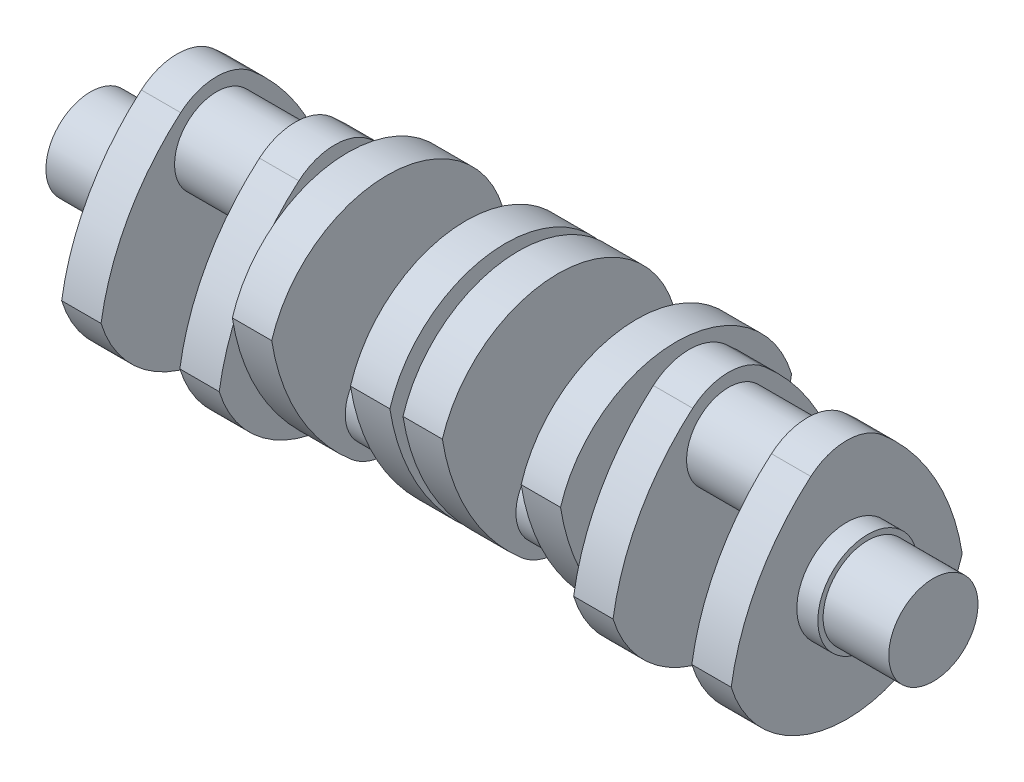
from build123d import *

# Parameters (mm, degrees)
END_JOURNAL_PROFILE_R         = 17
END_JOURNAL_34_DEPTH          = 25
SKETCH1_3_R                   = 19
JOURNAL_COLLAR_38_DEPTH       = 8
CRANK_WEB_1_DEPTH             = 15
CRANK_PIN_1_PROFILE_R         = 16
CRANK_PIN_1_32_DEPTH          = 15
MAIN_START                    = 5
MAIN_JOURNAL_SPACER_PROFILE_R = 17
MAIN_JOURNAL_SPACER_34_DEPTH  = 5
CRANK_WEB_3_DEPTH             = 15
CRANK_PIN_2_PROFILE_R         = 16
CRANK_PIN_2_32_DEPTH          = 30
CRANK_WEB_4_DEPTH             = 15
CENTRE_START                  = 2.5
CENTRE_JOURNAL_PROFILE_R      = 17
CENTRE_JOURNAL_HALF_34_DEPTH  = 2.5


with BuildPart() as part:
    # End Journal Profile → End Journal _34 (new body)
    with BuildSketch(Plane(origin=(0, 0, 0), x_dir=(0, 0, -1), z_dir=(1, 0, 0))):
        Circle(END_JOURNAL_PROFILE_R)
    extrude(amount=-END_JOURNAL_34_DEPTH)

    # Sketch1_3 → Journal Collar _38 (add)
    with BuildSketch(Plane(origin=(0, 0, 0), x_dir=(0, 0, -1), z_dir=(1, 0, 0))):
        Circle(SKETCH1_3_R)
    extrude(amount=JOURNAL_COLLAR_38_DEPTH)

    # Crank Web 1 Profile → Crank Web 1 (add)
    with BuildSketch(Plane(origin=(8, 0, 0), x_dir=(0, 0, -1), z_dir=(1, 0, 0))):
        with BuildLine():
            ThreePointArc((13.668094758, 40.943123461), (0, 46), (-13.668094758, 40.943123461))
            ThreePointArc((-13.668094758, 40.943123461), (-33.683444249, 16.469257624), (-44, -13.416407865))
            ThreePointArc((-44, -13.416407865), (0, -46), (44, -13.416407865))
            ThreePointArc((44, -13.416407865), (33.683444249, 16.469257624), (13.668094758, 40.943123461))
        make_face()
    crank_web_1 = extrude(amount=CRANK_WEB_1_DEPTH)

    # Crank Pin 1 Profile → Crank Pin 1 _32 (add)
    with BuildSketch(Plane(origin=(23, 0, 0), x_dir=(0, 0, -1), z_dir=(1, 0, 0))):
        with Locations(Location((0, 25, 0), (0, 0, 180))):
            Circle(CRANK_PIN_1_PROFILE_R)
    crank_pin_1_32 = extrude(amount=CRANK_PIN_1_32_DEPTH)

    # Crank Web 2 Mirror: Crank Web 1, Crank Pin 1 _32 across plane
    add(crank_web_1.mirror(Plane(origin=(38, 25, 0), x_dir=(0, 0, 1), z_dir=(1, 0, 0))))
    add(crank_pin_1_32.mirror(Plane(origin=(38, 25, 0), x_dir=(0, 0, 1), z_dir=(1, 0, 0))))

    # Main Journal Spacer Profile → Main Journal Spacer _34 (add)
    with BuildSketch(Plane(origin=(68, 0, 0), x_dir=(0, 0, -1), z_dir=(1, 0, 0)).offset(MAIN_START)):
        Circle(MAIN_JOURNAL_SPACER_PROFILE_R)
    extrude(amount=-MAIN_JOURNAL_SPACER_34_DEPTH)

    # Crank Web 3 Profile → Crank Web 3 (add)
    with BuildSketch(Plane(origin=(73, 0, 0), x_dir=(0, 0, -1), z_dir=(1, 0, 0))):
        with BuildLine():
            ThreePointArc((-13.668094758, -40.943123461), (0, -46), (13.668094758, -40.943123461))
            ThreePointArc((13.668094758, -40.943123461), (33.683444249, -16.469257624), (44, 13.416407865))
            ThreePointArc((44, 13.416407865), (0, 46), (-44, 13.416407865))
            ThreePointArc((-44, 13.416407865), (-33.683444249, -16.469257624), (-13.668094758, -40.943123461))
        make_face()
    extrude(amount=CRANK_WEB_3_DEPTH)

    # Crank Pin 2 Profile → Crank Pin 2 _32 (add)
    with BuildSketch(Plane(origin=(88, 0, 0), x_dir=(0, 0, -1), z_dir=(1, 0, 0))):
        with Locations((0, -25)):
            Circle(CRANK_PIN_2_PROFILE_R)
    extrude(amount=CRANK_PIN_2_32_DEPTH)

    # Crank Web 4 Profile → Crank Web 4 (add)
    with BuildSketch(Plane(origin=(118, 0, 0), x_dir=(0, 0, -1), z_dir=(1, 0, 0))):
        with BuildLine():
            ThreePointArc((-13.668094758, -40.943123461), (0, -46), (13.668094758, -40.943123461))
            ThreePointArc((13.668094758, -40.943123461), (33.683444249, -16.469257624), (44, 13.416407865))
            ThreePointArc((44, 13.416407865), (0, 46), (-44, 13.416407865))
            ThreePointArc((-44, 13.416407865), (-33.683444249, -16.469257624), (-13.668094758, -40.943123461))
        make_face()
    extrude(amount=CRANK_WEB_4_DEPTH)

    # Centre Journal Profile → Centre Journal Half _34 (add)
    with BuildSketch(Plane(origin=(133, 0, 0), x_dir=(0, 0, -1), z_dir=(1, 0, 0)).offset(CENTRE_START)):
        Circle(CENTRE_JOURNAL_PROFILE_R)
    extrude(amount=-CENTRE_JOURNAL_HALF_34_DEPTH)

    # Crankshaft Half Mirror: part across plane


with BuildPart() as part_1:
    add(part.part)
    add(part.part.mirror(Plane(origin=(135.5, 0, 0), x_dir=(0, 0, 1), z_dir=(1, 0, 0))))


solid = part_1.part
